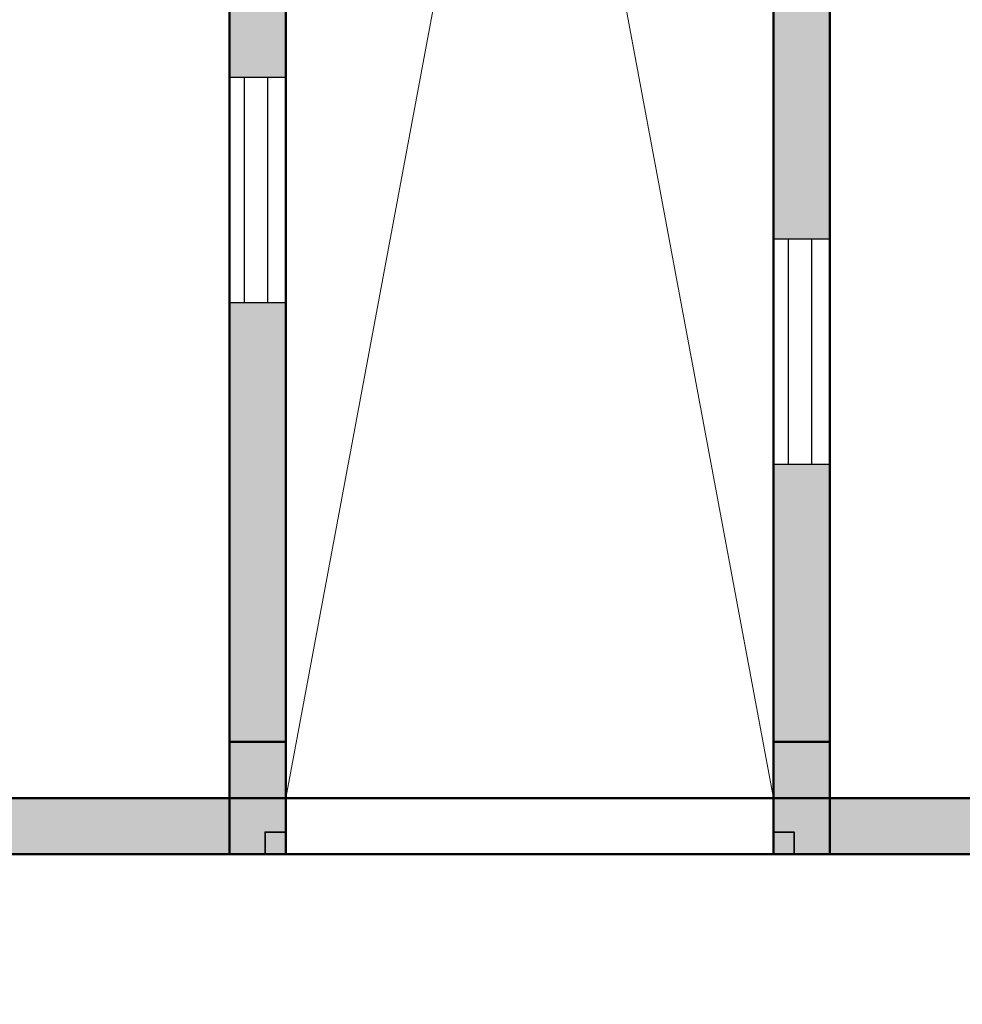
# Model space of a CAD drawing. Units: inches. Extents: x -7 to 1228, y -146 to 1091.
# Tile 20 of 88: x 513 to 664, y 36 to 194. Entities that reach past the tile are written whole.
import ezdxf

# ---------------------------------------------------------------- set-up
doc = ezdxf.new("R2010")
doc.units = ezdxf.units.IN
for name, color, linetype, lineweight in [('A-COLS', 6, 'Continuous', 35), ('A-FLOR-VOID', 7, 'Continuous', 18), ('A-GLAZ', 175, 'Continuous', 25), ('A-WALL', 7, 'Continuous', 50), ('A-WALL-PATT', 251, 'Continuous', 13)]:
    doc.layers.add(name, color=color, linetype=linetype, lineweight=lineweight)

# ---------------------------------------------------------------- blocks, each defined once
blk = doc.blocks.new('WIN-36')
for p, q in [((0, 36), (0, 0)), ((9, 36), (0, 36)), ((2.34, 36), (2.34, 0)), ((6.14, 0), (6.14, 36)), ((9, 0), (9, 36)), ((0, 0), (9, 0)), ((2.34, 0), (6.14, 0))]:
    blk.add_line(p, q)

msp = doc.modelspace()

# ---------------------------------------------------------------- hatches: boundary and pattern name
at = {"layer": 'A-COLS'}
h = msp.add_hatch(color=256, dxfattribs=at)
h.dxf.hatch_style = 1
h.paths.add_polyline_path([(556, 78), (547, 78), (547, 60), (552.71, 60), (552.71, 63.55), (556, 63.55)])
h = msp.add_hatch(color=256, dxfattribs=at)
h.dxf.hatch_style = 1
h.paths.add_polyline_path([(634, 63.55), (637.29, 63.55), (637.29, 60), (643, 60), (643, 78), (634, 78)])
h = msp.add_hatch(color=256, dxfattribs=at)
h.dxf.hatch_style = 1
h.paths.add_polyline_path([(552.71, 63.55), (552.71, 60), (556, 60), (556, 63.55)])
h = msp.add_hatch(color=256, dxfattribs=at)
h.dxf.hatch_style = 1
h.paths.add_polyline_path([(634, 63.55), (634, 60), (637.29, 60), (637.29, 63.55)])
at = {"layer": 'A-WALL-PATT'}
h = msp.add_hatch(color=256, dxfattribs=at)
h.dxf.hatch_style = 1
h.paths.add_polyline_path([(69, 568), (60, 568), (60, 493), (63.29, 493), (69, 493)])
h.paths.add_polyline_path([(69, 662.41), (60, 662.41), (60, 586), (69, 586)], flags=17)
h.paths.add_polyline_path([(69, 723), (184, 723), (184, 734), (179, 734), (179, 728), (69, 728), (69, 741.62), (60, 741.62), (60, 698.41), (69, 698.41)], flags=17)
h.paths.add_polyline_path([(69, 782), (231, 782), (231, 728), (231, 723), (231, 586), (236, 586), (236, 787), (69, 787), (69, 800.13), (60, 800.13), (60, 765.62), (69, 765.62)])
h.paths.add_polyline_path([(184, 842), (189, 842), (189, 848), (173, 848), (173, 842), (179, 842), (179, 787), (184, 787)])
h.paths.add_polyline_path([(118.22, 69), (69, 69), (69, 60), (118.22, 60)])
h.paths.add_polyline_path([(227, 69), (154.22, 69), (154.22, 60), (227, 60)])
h.paths.add_polyline_path([(236, 60), (232.71, 60), (227, 60), (227, 36), (236, 36)])
h.paths.add_polyline_path([(389, 60), (380, 60), (380, 36), (389, 36)])
h.paths.add_polyline_path([(384, 181), (380, 181), (380, 115), (380, 78), (384, 78)])
h.paths.add_polyline_path([(380, 115), (334.55, 115), (334.55, 109), (380, 109)])
h.paths.add_polyline_path([(274.55, 115), (236, 115), (236, 201), (232.71, 201), (231, 201), (231, 78), (236, 78), (236, 109), (274.55, 109)])
h.paths.add_polyline_path([(69, 123), (60, 123), (60, 78), (69, 78)])
h.paths.add_polyline_path([(69, 201), (60, 201), (60, 159), (69, 159)])
h.paths.add_polyline_path([(143, 219), (69, 219), (69, 213), (143, 213)], flags=17)
h.paths.add_polyline_path([(189, 219), (184, 219), (184, 274), (231, 274), (231, 219), (236, 219), (236, 279), (184, 279), (184, 297), (179, 297), (179, 279), (69, 279), (69, 290.91), (60, 290.91), (60, 262.18), (69, 262.18), (69, 274), (179, 274), (179, 219), (173, 219), (173, 213), (189, 213)])
h.paths.add_polyline_path([(69, 238.18), (60, 238.18), (60, 219), (69, 219)], flags=17)
h.paths.add_polyline_path([(69, 333), (60, 333), (60, 314.91), (69, 314.91), (69, 316.96)])
h.paths.add_polyline_path([(190, 338), (184, 338), (69, 338), (69, 333), (179, 333), (179, 327), (184, 327), (184, 333.02), (190, 333.05)])
h.paths.add_polyline_path([(69, 386.81), (60, 386.81), (60, 351), (69, 351)])
h.paths.add_polyline_path([(69, 475), (60, 475), (60, 422.81), (69, 422.81)])
h.paths.add_polyline_path([(236, 475), (231, 475), (231, 351.24), (236, 351.24)])
h.paths.add_polyline_path([(384, 475), (380, 475), (380, 362), (384, 362)])
h.paths.add_polyline_path([(547, 307), (439, 307), (439, 356), (445, 356), (445, 362), (433, 362), (433, 307), (380, 307), (380, 244), (380, 241), (384, 241), (384, 301), (433, 301), (433, 277), (439, 277), (439, 301), (547, 301)])
h.paths.add_polyline_path([(547, 241), (439, 241), (439, 247), (433, 247), (433, 235), (547, 235)])
h.paths.add_polyline_path([(450, 69), (440.29, 69), (424.89, 69), (389, 69), (389, 60), (450, 60)])
h.paths.add_polyline_path([(547, 69), (486, 69), (486, 60), (547, 60)])
h.paths.add_polyline_path([(556, 148.27), (547, 148.27), (547, 78), (556, 78)])
h.paths.add_polyline_path([(556, 223), (547, 223), (547, 195), (547, 184.27), (556, 184.27)])
h.paths.add_polyline_path([(556, 311.19), (547, 311.19), (547, 273.08), (556, 273.08)])
h.paths.add_polyline_path([(556, 344), (552.71, 344), (547, 344), (547, 335.19), (556, 335.19)])
h.paths.add_polyline_path([(556, 249.08), (547, 249.08), (547, 241), (556, 241)])
h.paths.add_polyline_path([(547, 362), (475, 362), (475, 356), (547, 356)], flags=0)
h.paths.add_polyline_path([(556, 399.62), (547, 399.62), (547, 362), (556, 362)])
h.paths.add_polyline_path([(556, 475), (547, 475), (547, 435.62), (556, 435.62)])
h.paths.add_polyline_path([(547, 493), (389, 493), (389, 487), (547, 487)])
h.paths.add_polyline_path([(380, 493), (278, 493), (278, 487), (380, 487)])
h.paths.add_polyline_path([(227, 493), (69, 493), (69, 487), (227, 487)])
h.paths.add_polyline_path([(643, 122.44), (634, 122.44), (634, 78), (643, 78)])
h.paths.add_polyline_path([(702.5, 69), (692.79, 69), (677.39, 69), (643, 69), (643, 60), (702.5, 60)])
h.paths.add_polyline_path([(798, 69), (738.5, 69), (738.5, 60), (798, 60)])
h.paths.add_polyline_path([(807, 60), (803.71, 60), (798, 60), (798, 36), (807, 36)])
h.paths.add_polyline_path([(807, 109), (846.75, 109), (846.75, 115), (807, 115), (807, 159), (802, 159), (802, 78), (807, 78)])
h.paths.add_polyline_path([(807, 201), (802, 201), (802, 195), (807, 195)])
h.paths.add_polyline_path([(643, 201), (634, 201), (634, 158.44), (643, 158.44)])
h.paths.add_polyline_path([(756, 225), (751, 225), (751, 219), (643, 219), (643, 213), (756, 213)])
h.paths.add_polyline_path([(643, 240.85), (634, 240.85), (634, 219), (643, 219)])
h.paths.add_polyline_path([(643, 274), (643, 288.63), (634, 288.63), (634, 264.85), (643, 264.85)])
h.paths.add_polyline_path([(802, 279), (756, 279), (756, 297), (751, 297), (751, 279), (643, 279), (643, 274), (751, 274), (751, 255), (756, 255), (756, 274), (802, 274)])
h.paths.add_polyline_path([(807, 333), (803.71, 333), (802, 333), (802, 279), (802, 274), (802, 219), (807, 219)])
h.paths.add_polyline_path([(956, 182), (951, 182), (951, 115), (906.75, 115), (906.75, 109), (951, 109), (951, 78), (956, 78)])
h.paths.add_polyline_path([(960, 60), (951, 60), (951, 36), (960, 36)])
h.paths.add_polyline_path([(1021, 69), (1005.78, 69), (960, 69), (960, 60), (1021, 60)])
h.paths.add_polyline_path([(956, 224), (951, 224), (951, 218), (956, 218)])
h.paths.add_polyline_path([(956, 302), (1004, 302), (1004, 278), (1010, 278), (1010, 302), (1118, 302), (1118, 290.81), (1127, 290.81), (1127, 326.97), (1118, 326.97), (1118, 320.97), (1118, 307), (1010, 307), (1010, 356), (1016, 356), (1016, 362), (1004, 362), (1004, 307), (951, 307), (951, 244), (951, 242), (954.29, 242), (956, 242)])
h.paths.add_polyline_path([(643, 333), (634, 333), (634, 312.63), (643, 312.63), (643, 316.96)])
h.paths.add_polyline_path([(756, 338), (643, 338), (643, 333), (751, 333), (751, 327), (756, 327)])
h.paths.add_polyline_path([(643, 388), (634, 388), (634, 351), (643, 351)])
h.paths.add_polyline_path([(807, 357), (802, 357), (802, 351), (807, 351)])
h.paths.add_polyline_path([(807, 475), (802, 475), (802, 393), (807, 393)])
h.paths.add_polyline_path([(643, 475), (634, 475), (634, 424), (643, 424)])
h.paths.add_polyline_path([(798, 493), (643, 493), (643, 487), (798, 487)])
h.paths.add_polyline_path([(634, 493), (556, 493), (556, 487), (634, 487)])
h.paths.add_polyline_path([(813, 493), (807, 493), (807, 487), (813, 487)])
h.paths.add_polyline_path([(951, 493), (849, 493), (849, 487), (951, 487)])
h.paths.add_polyline_path([(956, 484), (951, 484), (951, 374), (956, 374)])
h.paths.add_polyline_path([(1109, 493), (969, 493), (969, 487), (1109, 487)])
h.paths.add_polyline_path([(1127, 484), (1118, 484), (1118, 450.64), (1127, 450.64)])
h.paths.add_polyline_path([(1127, 414.64), (1118, 414.64), (1118, 365), (1127, 365)])
h.paths.add_polyline_path([(1109, 362), (1046, 362), (1046, 356), (1109, 356)], flags=17)
h.paths.add_polyline_path([(1127, 356), (1123.45, 356), (1118, 356), (1118, 350.97), (1127, 350.97)], flags=0)
h.paths.add_polyline_path([(1127, 266.81), (1118, 266.81), (1118, 262.36), (1118, 242), (1127, 242)], flags=17)
h.paths.add_polyline_path([(1118, 242), (1010, 242), (1010, 248), (1004, 248), (1004, 237), (1118, 237)])
h.paths.add_polyline_path([(1127, 224), (1118, 224), (1118, 170), (1127, 170)])
h.paths.add_polyline_path([(1127, 134), (1118, 134), (1118, 78), (1127, 78)])
h.paths.add_polyline_path([(1118, 69), (1057, 69), (1057, 60), (1118, 60)])
h.paths.add_polyline_path([(227, 571.55), (227, 574), (69, 574), (69, 568), (227, 568)])
h.paths.add_polyline_path([(380, 571.55), (380, 574), (278, 574), (278, 568), (380, 568)])
h.paths.add_polyline_path([(242, 574), (236, 574), (236, 568), (242, 568)])
h.paths.add_polyline_path([(547, 571.55), (547, 574), (389, 574), (389, 568), (547, 568)])
h.paths.add_polyline_path([(384, 733), (380, 733), (380, 586), (384, 586)])
h.paths.add_polyline_path([(556, 646), (634, 646), (634, 655), (547, 655), (547, 586), (556, 586)])
h.paths.add_polyline_path([(634, 574), (556, 574), (556, 568), (634, 568)])
h.paths.add_polyline_path([(643, 655), (634, 655), (634, 586), (643, 586)])
h.paths.add_polyline_path([(798, 574), (643, 574), (643, 568), (798, 568)])
h.paths.add_polyline_path([(643, 663.85), (634, 663.85), (634, 655), (643, 655)])
h.paths.add_polyline_path([(556, 676.97), (547, 676.97), (547, 655), (556, 655)])
h.paths.add_polyline_path([(556, 733), (547, 733), (547, 712.97), (556, 712.97)])
h.paths.add_polyline_path([(643, 710), (634, 710), (634, 699.85), (643, 699.85)])
h.paths.add_polyline_path([(807, 668), (802, 668), (802, 586), (807, 586)])
h.paths.add_polyline_path([(951, 574), (849, 574), (849, 568), (951, 568)])
h.paths.add_polyline_path([(956, 691), (951, 691), (951, 577), (956, 577)])
h.paths.add_polyline_path([(1109, 574), (969, 574), (969, 568), (1109, 568)])
h.paths.add_polyline_path([(1127, 643.4), (1118, 643.4), (1118, 577), (1127, 577)])
h.paths.add_polyline_path([(1127, 568), (1123.45, 568), (1118, 568), (1118, 493), (1127, 493)])
h.paths.add_polyline_path([(1127, 733), (1118, 733), (1118, 679.4), (1127, 679.4)])
h.paths.add_polyline_path([(1127, 777.35), (1118, 777.35), (1118, 770.04), (1118, 751), (1127, 751)], flags=17)
h.paths.add_polyline_path([(1118, 751), (1010, 751), (1010, 757), (1004, 757), (1004, 745), (1118, 745)])
h.paths.add_polyline_path([(956, 811), (1004, 811), (1004, 787), (1010, 787), (1010, 811), (1017.87, 811), (1017.87, 811.63, -0.414214), (1018.25, 812), (1031.98, 812, -0.414214), (1032.35, 811.63), (1032.35, 811), (1118, 811), (1118, 801.35), (1127, 801.35), (1127, 834.69), (1118, 834.69), (1118, 830.24), (1118, 817), (1010, 817), (1010, 866), (1016, 866), (1016, 872), (1004, 872), (1004, 817), (956, 817), (956, 866), (951, 866), (951, 751), (954.29, 751), (956, 751)])
h.paths.add_polyline_path([(1118, 872), (1046, 872), (1046, 866), (1118, 866)], flags=17)
h.paths.add_polyline_path([(1127, 924.71), (1118, 924.71), (1118, 884), (1127, 884)])
h.paths.add_polyline_path([(1127, 866), (1123.71, 866), (1118, 866), (1118, 858.69), (1127, 858.69)], flags=17)
h.paths.add_polyline_path([(956, 983), (951, 983), (951, 952), (807, 952), (807, 983), (802, 983), (802, 902), (807, 902), (807, 946), (951, 946), (951, 884), (956, 884)])
h.paths.add_polyline_path([(807, 842), (802, 842), (802, 787), (756, 787), (756, 806), (751, 806), (751, 787), (643, 787), (643, 782), (751, 782), (751, 764), (756, 764), (756, 782), (802, 782), (802, 728), (807, 728)])
h.paths.add_polyline_path([(756, 848), (643, 848), (643, 842), (751, 842), (751, 836), (756, 836)])
h.paths.add_polyline_path([(756, 734), (751, 734), (751, 728), (643, 728), (643, 723), (756, 723)])
h.paths.add_polyline_path([(643, 749.79), (634, 749.79), (634, 728), (637.29, 728), (643, 728)])
h.paths.add_polyline_path([(643, 805.41), (634, 805.41), (634, 773.79), (643, 773.79)])
h.paths.add_polyline_path([(643, 896.66), (634, 896.66), (634, 860), (637.29, 860), (643, 860)])
h.paths.add_polyline_path([(643, 842), (634, 842), (634, 829.41), (643, 829.41)])
h.paths.add_polyline_path([(643, 983), (634, 983), (634, 932.66), (643, 932.66)])
h.paths.add_polyline_path([(1127, 983), (1118, 983), (1118, 960.71), (1127, 960.71)])
h.paths.add_polyline_path([(1118, 1001), (1077.53, 1001), (1077.53, 992), (1118, 992)])
h.paths.add_polyline_path([(1041.53, 1001), (960, 1001), (960, 992), (1041.53, 992)])
h.paths.add_polyline_path([(960, 1025), (951, 1025), (951, 1001), (954.29, 1001), (960, 1001)])
h.paths.add_polyline_path([(807, 1025), (798, 1025), (798, 1001), (807, 1001)])
h.paths.add_polyline_path([(798, 1001), (738.5, 1001), (738.5, 992), (798, 992)])
h.paths.add_polyline_path([(702.5, 1001), (643, 1001), (643, 992), (702.5, 992)])
h.paths.add_polyline_path([(547, 1001), (499.11, 1001), (499.11, 992), (547, 992)])
h.paths.add_polyline_path([(463.11, 1001), (389, 1001), (389, 992), (463.11, 992)])
h.paths.add_polyline_path([(389, 1025), (380, 1025), (380, 1022), (380, 1001), (383.29, 1001), (389, 1001)])
h.paths.add_polyline_path([(236, 1025), (227, 1025), (227, 1001), (236, 1001)])
h.paths.add_polyline_path([(236, 983), (231, 983), (231, 860), (236, 860)])
h.paths.add_polyline_path([(274.55, 952), (236, 952), (236, 946), (274.55, 946)])
h.paths.add_polyline_path([(380, 952), (334.55, 952), (334.55, 946), (380, 946)])
h.paths.add_polyline_path([(384, 983), (380, 983), (380, 884), (383.29, 884), (384, 884)])
h.paths.add_polyline_path([(227, 1001), (155.01, 1001), (155.01, 992), (162.87, 992), (227, 992)])
h.paths.add_polyline_path([(119.01, 1001), (69, 1001), (69, 992), (119.01, 992)])
h.paths.add_polyline_path([(69, 983), (60, 983), (60, 922.99), (69, 922.99)])
h.paths.add_polyline_path([(69, 886.99), (60, 886.99), (60, 860), (63.29, 860), (69, 860)])
h.paths.add_polyline_path([(143, 848), (69, 848), (69, 842), (143, 842)])

# ---------------------------------------------------------------- linework, layer by layer
at = {"layer": 'A-COLS'}
for points in [[(556, 60), (552.71, 60), (552.71, 63.55), (556, 63.55)], [(634, 60), (637.29, 60), (637.29, 63.55), (634, 63.55)]]:
    msp.add_lwpolyline(points, close=True, dxfattribs=at)
at = {"layer": 'A-FLOR-VOID'}
for p, q in [((634, 487), (556, 69)), ((556, 487), (634, 69))]:
    msp.add_line(p, q, dxfattribs=at)
at = {"layer": 'A-WALL'}
for p, q in [((547, 493), (547, 60)), ((556, 493), (556, 60)), ((634, 493), (634, 60)), ((643, 493), (643, 60)), ((556, 60), (556, 406)), ((634, 60), (634, 406)), ((643, 60), (643, 213)), ((547, 60), (547, 189)), ((547, 60), (547, 78)), ((547, 78), (556, 78)), ((556, 78), (556, 60)), ((643, 78), (634, 78)), ((634, 78), (634, 60)), ((643, 60), (643, 78)), ((556, 69), (380, 69)), ((556, 69), (556, 60)), ((634, 69), (556, 69)), ((807, 69), (634, 69)), ((556, 60), (380, 60)), ((380, 60), (807, 60)), ((556, 60), (547, 60)), ((556, 60), (556, 60)), ((634, 60), (556, 60)), ((807, 60), (634, 60)), ((634, 60), (643, 60))]:
    msp.add_line(p, q, dxfattribs=at)

# ---------------------------------------------------------------- block references
at = {"layer": 'A-GLAZ'}
for p in [(547, 148.27), (634, 122.44)]:
    msp.add_blockref('WIN-36', p, dxfattribs=at)

doc.saveas('drawing.dxf')
